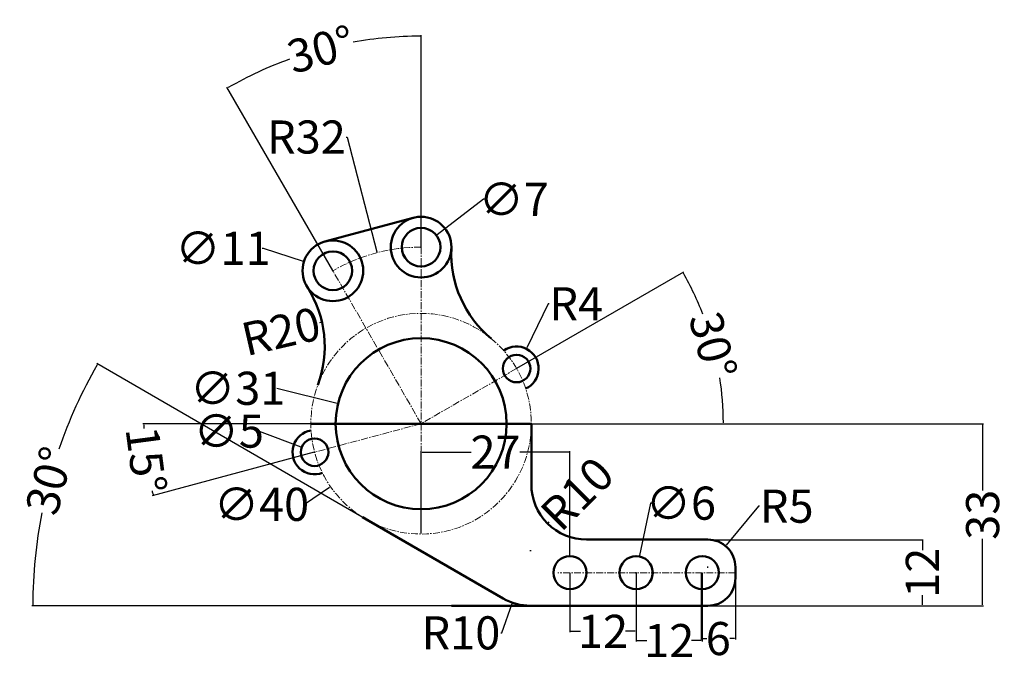
# Model space of a CAD drawing. Units: millimetres. Extents: x 90 to 269, y 31 to 148.
import ezdxf

# ---------------------------------------------------------------- set-up
doc = ezdxf.new("R2010")
doc.units = ezdxf.units.MM
doc.header["$MEASUREMENT"] = 0
doc.linetypes.add('CENTER', pattern=[2, 1.25, -0.25, 0.25, -0.25])
for name, color, linetype, lineweight in [('M-CNTR', 1, 'CENTER', 18), ('M-DIMS', 2, 'Continuous', 25), ('M-OUTL', 7, 'Continuous', 50)]:
    doc.layers.add(name, color=color, linetype=linetype, lineweight=lineweight)
doc.styles.get("Standard").update_dxf_attribs({"font": 'arial.ttf'})
doc.dimstyles.get("Standard").update_dxf_attribs({"dimtxt": 6, "dimasz": 0.18, "dimexe": 0.18, "dimexo": 0.0625, "dimgap": 0.09, "dimtad": 0, "dimtoh": 1, "dimdec": 0, "dimzin": 0, "dimdsep": 46, "dimtxsty": 'Standard', "dimcen": 0.09, "dimadec": 0, "dimazin": 0, "dimtfac": 1, "dimtdec": 0, "dimtofl": 0, "dimtmove": 0, "dimatfit": 3, "dimfxl": 1, "dimtolj": 1, "dimtzin": 0, "dimarcsym": 0})

# ---------------------------------------------------------------- blocks, each defined once
blk = doc.blocks.new('*D1')
at = {"layer": 'Defpoints', "color": 0, "transparency": 16777216}
for p in [(178.24, 74.72), (178.24, 41.72), (264.58, 41.72)]:
    blk.add_point(p, dxfattribs=at)
at = {"layer": 'M-DIMS', "color": 0, "lineweight": -2, "transparency": 16777216}
for p, q in [((178.3, 74.72), (264.76, 74.72)), ((264.58, 74.54), (264.58, 62.61)), ((264.58, 41.9), (264.58, 53.84)), ((178.3, 41.72), (264.76, 41.72))]:
    blk.add_line(p, q, dxfattribs=at)
at = {"layer": 'M-DIMS', "color": 0, "transparency": 16777216}
for points in [[(264.55, 74.54), (264.61, 74.54), (264.58, 74.72)], [(264.55, 41.9), (264.61, 41.9), (264.58, 41.72)]]:
    blk.add_solid(points, dxfattribs=at)
at = {"layer": 'M-DIMS', "color": 0, "transparency": 16777216, "insert": (264.58, 58.22), "char_height": 6, "attachment_point": 5, "rotation": 90}
blk.add_mtext('\\A1;33', dxfattribs=at)
blk = doc.blocks.new('*D2')
at = {"layer": 'Defpoints', "color": 0, "transparency": 16777216}
for p in [(215.42, 53.68), (215.42, 41.72), (253.65, 41.72)]:
    blk.add_point(p, dxfattribs=at)
at = {"layer": 'M-DIMS', "color": 0, "lineweight": -2, "transparency": 16777216}
for p, q in [((215.48, 53.68), (253.83, 53.68)), ((253.65, 53.5), (253.65, 51.77)), ((253.65, 41.9), (253.65, 43.63)), ((215.48, 41.72), (253.83, 41.72))]:
    blk.add_line(p, q, dxfattribs=at)
at = {"layer": 'M-DIMS', "color": 0, "transparency": 16777216}
for points in [[(253.62, 53.5), (253.68, 53.5), (253.65, 53.68)], [(253.62, 41.9), (253.68, 41.9), (253.65, 41.72)]]:
    blk.add_solid(points, dxfattribs=at)
at = {"layer": 'M-DIMS', "color": 0, "transparency": 16777216, "insert": (253.65, 47.7), "char_height": 6, "attachment_point": 5, "rotation": 90}
blk.add_mtext('\\A1;12', dxfattribs=at)
blk = doc.blocks.new('*D3')
at = {"layer": 'Defpoints', "color": 0, "transparency": 16777216}
for p in [(217.93, 52.57), (214.74, 48.72)]:
    blk.add_point(p, dxfattribs=at)
at = {"layer": 'M-DIMS', "color": 0, "lineweight": -2, "transparency": 16777216}
for p, q in [((223.93, 59.77), (218.05, 52.71)), ((224.11, 59.77), (223.93, 59.77)), ((214.65, 48.72), (214.83, 48.72)), ((214.74, 48.63), (214.74, 48.81))]:
    blk.add_line(p, q, dxfattribs=at)
at = {"layer": 'M-DIMS', "color": 0, "transparency": 16777216}
blk.add_solid([(218.03, 52.73), (218.07, 52.69), (217.93, 52.57)], dxfattribs=at)
at = {"layer": 'M-DIMS', "color": 0, "transparency": 16777216, "insert": (229.06, 59.77), "char_height": 6, "attachment_point": 5}
blk.add_mtext('\\A1;R5', dxfattribs=at)
blk = doc.blocks.new('*D4')
at = {"layer": 'Defpoints', "color": 0, "transparency": 16777216}
for p in [(181.82, 88.32), (180.06, 84.72)]:
    blk.add_point(p, dxfattribs=at)
at = {"layer": 'M-DIMS', "color": 0, "lineweight": -2, "transparency": 16777216}
for p, q in [((185.8, 96.45), (181.9, 88.48)), ((185.98, 96.45), (185.8, 96.45)), ((179.97, 84.72), (180.15, 84.72)), ((180.06, 84.63), (180.06, 84.81))]:
    blk.add_line(p, q, dxfattribs=at)
at = {"layer": 'M-DIMS', "color": 0, "transparency": 16777216}
blk.add_solid([(181.87, 88.49), (181.92, 88.46), (181.82, 88.32)], dxfattribs=at)
at = {"layer": 'M-DIMS', "color": 0, "transparency": 16777216, "insert": (190.89, 96.45), "char_height": 6, "attachment_point": 5}
blk.add_mtext('\\A1;R4', dxfattribs=at)
blk = doc.blocks.new('*D5')
at = {"layer": 'Defpoints', "color": 0, "transparency": 16777216}
for p in [(154.75, 105.71), (162.74, 74.72)]:
    blk.add_point(p, dxfattribs=at)
at = {"layer": 'M-DIMS', "color": 0, "lineweight": -2, "transparency": 16777216}
for p, q in [((149.17, 126.68), (149.35, 126.68)), ((149.35, 126.68), (154.71, 105.89)), ((162.65, 74.72), (162.83, 74.72)), ((162.74, 74.63), (162.74, 74.81))]:
    blk.add_line(p, q, dxfattribs=at)
at = {"layer": 'M-DIMS', "color": 0, "transparency": 16777216}
blk.add_solid([(154.74, 105.89), (154.68, 105.88), (154.75, 105.71)], dxfattribs=at)
at = {"layer": 'M-DIMS', "color": 0, "transparency": 16777216, "insert": (141.94, 126.68), "char_height": 6, "attachment_point": 5}
blk.add_mtext('\\A1;R32', dxfattribs=at)
blk = doc.blocks.new('*D6')
at = {"layer": 'Defpoints', "color": 0, "transparency": 16777216}
for p in [(192.74, 63.72), (185.67, 56.65)]:
    blk.add_point(p, dxfattribs=at)
at = {"layer": 'M-DIMS', "color": 0, "lineweight": -2, "transparency": 16777216}
blk.add_line((185.92, 56.91), (185.79, 56.78), dxfattribs=at)
at = {"layer": 'M-DIMS', "color": 0, "transparency": 16777216}
blk.add_solid([(185.77, 56.8), (185.81, 56.76), (185.67, 56.65)], dxfattribs=at)
at = {"layer": 'M-DIMS', "color": 0, "transparency": 16777216, "insert": (191.05, 62.03), "char_height": 6, "attachment_point": 5, "rotation": 45}
blk.add_mtext('\\A1;R10', dxfattribs=at)
blk = doc.blocks.new('*D7')
at = {"layer": 'Defpoints', "color": 0, "transparency": 16777216}
for p in [(182.6, 51.72), (179.3, 42.28)]:
    blk.add_point(p, dxfattribs=at)
at = {"layer": 'M-DIMS', "color": 0, "lineweight": -2, "transparency": 16777216}
for p, q in [((182.6, 51.63), (182.6, 51.81)), ((182.51, 51.72), (182.69, 51.72)), ((177.39, 36.81), (179.24, 42.11)), ((177.21, 36.81), (177.39, 36.81))]:
    blk.add_line(p, q, dxfattribs=at)
at = {"layer": 'M-DIMS', "color": 0, "transparency": 16777216}
blk.add_solid([(179.21, 42.12), (179.27, 42.1), (179.3, 42.28)], dxfattribs=at)
at = {"layer": 'M-DIMS', "color": 0, "transparency": 16777216, "insert": (169.96, 36.81), "char_height": 6, "attachment_point": 5}
blk.add_mtext('\\A1;R10', dxfattribs=at)
blk = doc.blocks.new('*D8')
at = {"layer": 'Defpoints', "color": 0, "transparency": 16777216}
for p in [(189.74, 69.57), (162.74, 54.72), (189.74, 50.72)]:
    blk.add_point(p, dxfattribs=at)
at = {"layer": 'M-DIMS', "color": 0, "lineweight": -2, "transparency": 16777216}
for p, q in [((162.74, 54.79), (162.74, 69.75)), ((189.74, 50.79), (189.74, 69.75)), ((162.92, 69.57), (171.8, 69.57)), ((189.56, 69.57), (180.67, 69.57))]:
    blk.add_line(p, q, dxfattribs=at)
at = {"layer": 'M-DIMS', "color": 0, "transparency": 16777216}
for points in [[(162.92, 69.6), (162.92, 69.54), (162.74, 69.57)], [(189.56, 69.6), (189.56, 69.54), (189.74, 69.57)]]:
    blk.add_solid(points, dxfattribs=at)
at = {"layer": 'M-DIMS', "color": 0, "transparency": 16777216, "insert": (176.24, 69.57), "char_height": 6, "attachment_point": 5}
blk.add_mtext('\\A1;27', dxfattribs=at)
blk = doc.blocks.new('*D9')
at = {"layer": 'Defpoints', "color": 0, "transparency": 16777216}
for p in [(189.74, 47.72), (201.74, 47.72), (201.74, 37.09)]:
    blk.add_point(p, dxfattribs=at)
at = {"layer": 'M-DIMS', "color": 0, "lineweight": -2, "transparency": 16777216}
for p, q in [((189.74, 47.66), (189.74, 36.91)), ((201.74, 47.66), (201.74, 36.91)), ((189.92, 37.09), (191.66, 37.09)), ((201.56, 37.09), (199.81, 37.09))]:
    blk.add_line(p, q, dxfattribs=at)
at = {"layer": 'M-DIMS', "color": 0, "transparency": 16777216}
for points in [[(189.92, 37.12), (189.92, 37.06), (189.74, 37.09)], [(201.56, 37.12), (201.56, 37.06), (201.74, 37.09)]]:
    blk.add_solid(points, dxfattribs=at)
at = {"layer": 'M-DIMS', "color": 0, "transparency": 16777216, "insert": (195.74, 37.09), "char_height": 6, "attachment_point": 5}
blk.add_mtext('\\A1;12', dxfattribs=at)
blk = doc.blocks.new('*D10')
at = {"layer": 'Defpoints', "color": 0, "transparency": 16777216}
for p in [(201.74, 47.72), (213.74, 47.72), (213.74, 35.41)]:
    blk.add_point(p, dxfattribs=at)
at = {"layer": 'M-DIMS', "color": 0, "lineweight": -2, "transparency": 16777216}
for p, q in [((201.74, 47.66), (201.74, 35.23)), ((213.74, 47.66), (213.74, 35.23)), ((201.92, 35.41), (203.66, 35.41)), ((213.56, 35.41), (211.81, 35.41))]:
    blk.add_line(p, q, dxfattribs=at)
at = {"layer": 'M-DIMS', "color": 0, "transparency": 16777216}
for points in [[(201.92, 35.44), (201.92, 35.38), (201.74, 35.41)], [(213.56, 35.44), (213.56, 35.38), (213.74, 35.41)]]:
    blk.add_solid(points, dxfattribs=at)
at = {"layer": 'M-DIMS', "color": 0, "transparency": 16777216, "insert": (207.74, 35.41), "char_height": 6, "attachment_point": 5}
blk.add_mtext('\\A1;12', dxfattribs=at)
blk = doc.blocks.new('*D11')
at = {"layer": 'Defpoints', "color": 0, "transparency": 16777216}
for p in [(213.55, 47.72), (219.74, 47.72), (219.74, 35.78)]:
    blk.add_point(p, dxfattribs=at)
at = {"layer": 'M-DIMS', "color": 0, "lineweight": -2, "transparency": 16777216}
for p, q in [((213.55, 47.66), (213.55, 35.6)), ((219.74, 47.66), (219.74, 35.6)), ((213.73, 35.78), (214.57, 35.78)), ((219.56, 35.78), (218.72, 35.78))]:
    blk.add_line(p, q, dxfattribs=at)
at = {"layer": 'M-DIMS', "color": 0, "transparency": 16777216}
for points in [[(213.73, 35.81), (213.73, 35.75), (213.55, 35.78)], [(219.56, 35.81), (219.56, 35.75), (219.74, 35.78)]]:
    blk.add_solid(points, dxfattribs=at)
at = {"layer": 'M-DIMS', "color": 0, "transparency": 16777216, "insert": (216.64, 35.78), "char_height": 6, "attachment_point": 5}
blk.add_mtext('\\A1;6', dxfattribs=at)
blk = doc.blocks.new('*D12')
at = {"layer": 'Defpoints', "color": 0, "transparency": 16777216}
for p in [(141.5, 104.12), (151.97, 100.75)]:
    blk.add_point(p, dxfattribs=at)
at = {"layer": 'M-DIMS', "color": 0, "lineweight": -2, "transparency": 16777216}
for p, q in [((133.89, 106.51), (134.07, 106.51)), ((134.07, 106.51), (141.33, 104.17)), ((146.65, 102.44), (146.83, 102.44)), ((146.74, 102.35), (146.74, 102.53))]:
    blk.add_line(p, q, dxfattribs=at)
at = {"layer": 'M-DIMS', "color": 0, "transparency": 16777216}
blk.add_solid([(141.34, 104.2), (141.32, 104.14), (141.5, 104.12)], dxfattribs=at)
at = {"layer": 'M-DIMS', "color": 0, "transparency": 16777216, "insert": (126.81, 106.51), "char_height": 6, "attachment_point": 5}
blk.add_mtext('\\A1;∅11', dxfattribs=at)
blk = doc.blocks.new('*D13')
at = {"layer": 'Defpoints', "color": 0, "transparency": 16777216}
for p in [(165.52, 108.85), (159.96, 104.6)]:
    blk.add_point(p, dxfattribs=at)
at = {"layer": 'M-DIMS', "color": 0, "lineweight": -2, "transparency": 16777216}
for p, q in [((174.06, 115.39), (165.66, 108.96)), ((174.24, 115.39), (174.06, 115.39)), ((162.65, 106.72), (162.83, 106.72)), ((162.74, 106.63), (162.74, 106.81))]:
    blk.add_line(p, q, dxfattribs=at)
at = {"layer": 'M-DIMS', "color": 0, "transparency": 16777216}
blk.add_solid([(165.64, 108.98), (165.68, 108.94), (165.52, 108.85)], dxfattribs=at)
at = {"layer": 'M-DIMS', "color": 0, "transparency": 16777216, "insert": (179.56, 115.39), "char_height": 6, "attachment_point": 5}
blk.add_mtext('\\A1;∅7', dxfattribs=at)
blk = doc.blocks.new('*D14')
at = {"layer": 'Defpoints', "color": 0, "transparency": 16777216}
for p in [(141.08, 70.44), (145.75, 68.65)]:
    blk.add_point(p, dxfattribs=at)
at = {"layer": 'M-DIMS', "color": 0, "lineweight": -2, "transparency": 16777216}
for p, q in [((133.21, 73.38), (133.39, 73.38)), ((133.39, 73.38), (140.91, 70.5)), ((143.33, 69.55), (143.51, 69.55)), ((143.42, 69.46), (143.42, 69.64))]:
    blk.add_line(p, q, dxfattribs=at)
at = {"layer": 'M-DIMS', "color": 0, "transparency": 16777216}
blk.add_solid([(140.93, 70.53), (140.9, 70.48), (141.08, 70.44)], dxfattribs=at)
at = {"layer": 'M-DIMS', "color": 0, "transparency": 16777216, "insert": (127.87, 73.38), "char_height": 6, "attachment_point": 5}
blk.add_mtext('\\A1;∅5', dxfattribs=at)
blk = doc.blocks.new('*D15')
at = {"layer": 'Defpoints', "color": 0, "transparency": 16777216}
for p in [(147.68, 78.41), (177.79, 71.03)]:
    blk.add_point(p, dxfattribs=at)
at = {"layer": 'M-DIMS', "color": 0, "lineweight": -2, "transparency": 16777216}
for p, q in [((136.55, 81.14), (147.51, 78.46)), ((162.65, 74.72), (162.83, 74.72)), ((162.74, 74.63), (162.74, 74.81))]:
    blk.add_line(p, q, dxfattribs=at)
at = {"layer": 'M-DIMS', "color": 0, "transparency": 16777216}
blk.add_solid([(147.51, 78.49), (147.5, 78.43), (147.68, 78.41)], dxfattribs=at)
at = {"layer": 'M-DIMS', "color": 0, "transparency": 16777216, "insert": (129.48, 81.14), "char_height": 6, "attachment_point": 5}
blk.add_mtext('\\A1;∅31', dxfattribs=at)
blk = doc.blocks.new('*D16')
at = {"layer": 'Defpoints', "color": 0, "transparency": 16777216}
for p in [(144.75, 93.16), (125.26, 88.7)]:
    blk.add_point(p, dxfattribs=at)
at = {"layer": 'M-DIMS', "color": 0, "lineweight": -2, "transparency": 16777216}
blk.add_line((144.4, 93.08), (144.58, 93.12), dxfattribs=at)
at = {"layer": 'M-DIMS', "color": 0, "transparency": 16777216}
blk.add_solid([(144.57, 93.15), (144.58, 93.09), (144.75, 93.16)], dxfattribs=at)
at = {"layer": 'M-DIMS', "color": 0, "transparency": 16777216, "insert": (137.33, 91.46), "char_height": 6, "attachment_point": 5, "rotation": 12.8998}
blk.add_mtext('\\A1;R20', dxfattribs=at)
blk = doc.blocks.new('*D17')
at = {"layer": 'Defpoints', "color": 0, "transparency": 16777216}
for p in [(179.18, 86.11), (146.29, 63.34)]:
    blk.add_point(p, dxfattribs=at)
at = {"layer": 'M-DIMS', "color": 0, "lineweight": -2, "transparency": 16777216}
for p, q in [((162.65, 74.72), (162.83, 74.72)), ((162.74, 74.63), (162.74, 74.81)), ((141.62, 60.11), (146.14, 63.24)), ((141.44, 60.11), (141.62, 60.11))]:
    blk.add_line(p, q, dxfattribs=at)
at = {"layer": 'M-DIMS', "color": 0, "transparency": 16777216}
blk.add_solid([(146.13, 63.26), (146.16, 63.21), (146.29, 63.34)], dxfattribs=at)
at = {"layer": 'M-DIMS', "color": 0, "transparency": 16777216, "insert": (133.8, 60.11), "char_height": 6, "attachment_point": 5}
blk.add_mtext('\\A1;∅40', dxfattribs=at)
blk = doc.blocks.new('*D18')
at = {"layer": 'Defpoints', "color": 0, "transparency": 16777216}
for p in [(150.54, 143.9), (162.74, 106.72), (146.74, 102.44), (162.74, 74.72), (162.74, 54.72)]:
    blk.add_point(p, dxfattribs=at)
at = {"layer": 'M-DIMS', "color": 0, "lineweight": -2, "transparency": 16777216}
for p, q in [((162.74, 106.79), (162.74, 145.14)), ((146.71, 102.49), (127.53, 135.71))]:
    blk.add_line(p, q, dxfattribs=at)
for start, end in [(90.1468, 100.1216), (109.8784, 119.8532)]:
    blk.add_arc((162.74, 74.72), 70.24, start, end, dxfattribs=at)
at = {"layer": 'M-DIMS', "color": 0, "transparency": 16777216}
for points in [[(162.56, 144.99), (162.56, 144.93), (162.74, 144.96)], [(127.79, 135.62), (127.76, 135.67), (127.62, 135.55)]]:
    blk.add_solid(points, dxfattribs=at)
at = {"layer": 'M-DIMS', "color": 0, "transparency": 16777216, "insert": (144.56, 142.57), "char_height": 6, "attachment_point": 5, "rotation": 15}
blk.add_mtext('\\A1;30°', dxfattribs=at)
blk = doc.blocks.new('*D19')
at = {"layer": 'Defpoints', "color": 0, "transparency": 16777216}
for p in [(97.61, 71.68), (152.13, 57.77), (177.6, 43.06), (168.25, 41.72), (182.6, 41.72)]:
    blk.add_point(p, dxfattribs=at)
at = {"layer": 'M-DIMS', "color": 0, "lineweight": -2, "transparency": 16777216}
for p, q in [((152.07, 57.8), (103.9, 85.61)), ((168.19, 41.72), (92.14, 41.72))]:
    blk.add_line(p, q, dxfattribs=at)
for start, end in [(150.1177, 161.0898), (168.9102, 179.8823)]:
    blk.add_arc((179.92, 41.72), 87.6, start, end, dxfattribs=at)
at = {"layer": 'M-DIMS', "color": 0, "transparency": 16777216}
for points in [[(103.94, 85.38), (104, 85.35), (104.06, 85.52)], [(92.35, 41.9), (92.29, 41.9), (92.32, 41.72)]]:
    blk.add_solid(points, dxfattribs=at)
at = {"layer": 'M-DIMS', "color": 0, "transparency": 16777216, "insert": (95.31, 64.4), "char_height": 6, "attachment_point": 5, "rotation": 75}
blk.add_mtext('\\A1;30°', dxfattribs=at)
blk = doc.blocks.new('*D20')
at = {"layer": 'Defpoints', "color": 0, "transparency": 16777216}
for p in [(142.74, 74.72), (162.74, 74.72), (182.74, 74.72), (112.64, 70.34), (143.42, 69.55)]:
    blk.add_point(p, dxfattribs=at)
at = {"layer": 'M-DIMS', "color": 0, "lineweight": -2, "transparency": 16777216}
for p, q in [((142.67, 74.72), (112.27, 74.72)), ((143.36, 69.53), (113.99, 61.66))]:
    blk.add_line(p, q, dxfattribs=at)
for start, end in [(180.2051, 180.9995), (194.0005, 194.7949)]:
    blk.add_arc((162.74, 74.72), 50.29, start, end, dxfattribs=at)
at = {"layer": 'M-DIMS', "color": 0, "transparency": 16777216}
for points in [[(112.42, 74.54), (112.48, 74.54), (112.45, 74.72)], [(114.15, 61.89), (114.09, 61.88), (114.16, 61.71)]]:
    blk.add_solid(points, dxfattribs=at)
at = {"layer": 'M-DIMS', "color": 0, "transparency": 16777216, "insert": (112.88, 68.16), "char_height": 6, "attachment_point": 5, "rotation": 277.5}
blk.add_mtext('\\A1;15°', dxfattribs=at)
blk = doc.blocks.new('*D21')
at = {"layer": 'Defpoints', "color": 0, "transparency": 16777216}
for p in [(180.06, 84.72), (216.73, 84.24), (142.74, 74.72), (162.74, 74.72), (182.74, 74.72)]:
    blk.add_point(p, dxfattribs=at)
at = {"layer": 'M-DIMS', "color": 0, "lineweight": -2, "transparency": 16777216}
for p, q in [((180.11, 84.76), (210.37, 102.23)), ((182.8, 74.72), (217.74, 74.72))]:
    blk.add_line(p, q, dxfattribs=at)
for start, end in [(21.2551, 29.8119), (0.1881, 8.7449)]:
    blk.add_arc((162.74, 74.72), 54.82, start, end, dxfattribs=at)
at = {"layer": 'M-DIMS', "color": 0, "transparency": 16777216}
for points in [[(210.28, 101.96), (210.33, 101.99), (210.21, 102.14)], [(217.59, 74.9), (217.53, 74.9), (217.56, 74.72)]]:
    blk.add_solid(points, dxfattribs=at)
at = {"layer": 'M-DIMS', "color": 0, "transparency": 16777216, "insert": (215.69, 88.91), "char_height": 6, "attachment_point": 5, "rotation": 285}
blk.add_mtext('\\A1;30°', dxfattribs=at)
blk = doc.blocks.new('*D22')
at = {"layer": 'Defpoints', "color": 0, "transparency": 16777216}
for p in [(202.35, 50.66), (201.13, 44.79)]:
    blk.add_point(p, dxfattribs=at)
at = {"layer": 'M-DIMS', "color": 0, "lineweight": -2, "transparency": 16777216}
for p, q in [((204.36, 60.32), (202.38, 50.84)), ((204.54, 60.32), (204.36, 60.32)), ((201.65, 47.72), (201.83, 47.72)), ((201.74, 47.63), (201.74, 47.81))]:
    blk.add_line(p, q, dxfattribs=at)
at = {"layer": 'M-DIMS', "color": 0, "transparency": 16777216}
blk.add_solid([(202.35, 50.84), (202.41, 50.83), (202.35, 50.66)], dxfattribs=at)
at = {"layer": 'M-DIMS', "color": 0, "transparency": 16777216, "insert": (209.86, 60.32), "char_height": 6, "attachment_point": 5}
blk.add_mtext('\\A1;∅6', dxfattribs=at)

msp = doc.modelspace()

# ---------------------------------------------------------------- linework, layer by layer
at = {"layer": 'M-CNTR'}
for p, q in [((162.74, 74.72), (143.42, 69.55)), ((219.74, 47.72), (187.54, 47.72))]:
    msp.add_line(p, q, dxfattribs=at)
msp.add_lwpolyline([(180.06, 84.72), (162.74, 74.72), (146.74, 102.44, -0.131652), (162.74, 106.72), (162.74, 54.72)], format="xyb", dxfattribs=at)
msp.add_circle((162.74, 74.72), 20, dxfattribs=at)
at = {"layer": 'M-OUTL'}
msp.add_line((145.31, 107.75), (161.31, 112.04), dxfattribs=at)
for points in [[(142.74, 74.72), (182.74, 74.72), (182.74, 63.72, 0.414214), (192.74, 53.72), (214.74, 53.72, -0.414214), (219.74, 48.72), (219.74, 46.72, -0.414214), (214.74, 41.72), (182.6, 41.72)], [(152.13, 57.77), (177.6, 43.06, 0.131652), (182.6, 41.72), (168.25, 41.72)]]:
    msp.add_lwpolyline(points, format="xyb", dxfattribs=at)
msp.add_lwpolyline([(152.35, 57.63), (153.13, 57.18)], dxfattribs=at)
for centre, radius in [((162.74, 106.72), 5.5), ((162.74, 106.72), 3.5), ((146.74, 102.44), 5.5), ((146.74, 102.44), 3.5), ((162.74, 74.72), 15.5), ((180.06, 84.72), 2.5), ((143.42, 69.55), 2.5), ((189.74, 47.72), 3), ((201.74, 47.72), 3), ((213.74, 47.72), 3)]:
    msp.add_circle(centre, radius, dxfattribs=at)
for centre, radius, start, end in [((188.21, 105.56), 20, 177.3924, 230.4434), ((125.26, 88.7), 20, 339.5566, 32.6076), ((180.06, 84.72), 4, 294.2608, 125.7392), ((143.42, 69.55), 4, 99.2608, 290.7392)]:
    msp.add_arc(centre, radius, start, end, dxfattribs=at)

# ---------------------------------------------------------------- dimensions: what is measured, and where the dimension line sits
at = {"layer": 'M-DIMS'}
for base, line1, line2, picture, middle in [((150.54, 143.9), ((162.74, 106.72), (162.74, 54.72)), ((162.74, 74.72), (146.74, 102.44)), '*D18', (144.56, 142.57)), ((216.73, 84.24), ((142.74, 74.72), (182.74, 74.72)), ((180.06, 84.72), (162.74, 74.72)), '*D21', (215.69, 88.91)), ((97.61, 71.68), ((182.6, 41.72), (168.25, 41.72)), ((152.13, 57.77), (177.6, 43.06)), '*D19', (95.31, 64.4)), ((112.64, 70.34), ((162.74, 74.72), (143.42, 69.55)), ((142.74, 74.72), (182.74, 74.72)), '*D20', (112.88, 68.16))]:
    dim = msp.add_angular_dim_2l(base=base, line1=line1, line2=line2, dimstyle='Standard', override={"dimclrd": 0, "dimclre": 0, "dimclrt": 0}, dxfattribs=at)
    dim.commit()
    dim.dimension.update_dxf_attribs({"geometry": picture, "text_midpoint": middle})
for center, mpoint, picture, middle in [((162.74, 74.72), (154.75, 105.71), '*D5', (141.94, 126.68)), ((180.06, 84.72), (181.82, 88.32), '*D4', (190.89, 96.45)), ((125.26, 88.7), (144.75, 93.16), '*D16', (137.33, 91.46)), ((192.74, 63.72), (185.67, 56.65), '*D6', (191.05, 62.03)), ((214.74, 48.72), (217.93, 52.57), '*D3', (229.06, 59.77)), ((182.6, 51.72), (179.3, 42.28), '*D7', (169.96, 36.81))]:
    dim = msp.add_radius_dim(center=center, mpoint=mpoint, dimstyle='Standard', override={"dimclrd": 0, "dimclre": 0, "dimclrt": 0}, dxfattribs=at)
    dim.commit()
    dim.dimension.update_dxf_attribs({"geometry": picture, "text_midpoint": middle, "dimtype": 164})
for p1, p2, picture, middle in [((159.96, 104.6), (165.52, 108.85), '*D13', (179.56, 115.39)), ((151.97, 100.75), (141.5, 104.12), '*D12', (126.81, 106.51)), ((179.18, 86.11), (146.29, 63.34), '*D17', (133.8, 60.11)), ((177.79, 71.03), (147.68, 78.41), '*D15', (136.55, 81.14)), ((145.75, 68.65), (141.08, 70.44), '*D14', (127.87, 73.38)), ((201.13, 44.79), (202.35, 50.66), '*D22', (209.86, 60.32))]:
    dim = msp.add_diameter_dim_2p(p1=p1, p2=p2, dimstyle='Standard', override={"dimclrd": 0, "dimclre": 0, "dimclrt": 0}, dxfattribs=at)
    dim.commit()
    dim.dimension.update_dxf_attribs({"geometry": picture, "text_midpoint": middle, "dimtype": 163})
for base, p1, p2, picture, middle in [((189.74, 69.57), (162.74, 54.72), (189.74, 50.72), '*D8', (176.24, 69.57)), ((201.74, 37.09), (189.74, 47.72), (201.74, 47.72), '*D9', (195.74, 37.09)), ((213.74, 35.41), (201.74, 47.72), (213.74, 47.72), '*D10', (207.74, 35.41)), ((219.74, 35.78), (213.55, 47.72), (219.74, 47.72), '*D11', (216.64, 35.78))]:
    dim = msp.add_linear_dim(base=base, p1=p1, p2=p2, dimstyle='Standard', override={"dimclrd": 0, "dimclre": 0, "dimclrt": 0}, dxfattribs=at)
    dim.commit()
    dim.dimension.update_dxf_attribs({"geometry": picture, "text_midpoint": middle})
for base, p1, p2, picture, middle in [((264.58, 41.72), (178.24, 74.72), (178.24, 41.72), '*D1', (264.58, 58.22)), ((253.65, 41.72), (215.42, 53.68), (215.42, 41.72), '*D2', (253.65, 47.7))]:
    dim = msp.add_linear_dim(base=base, p1=p1, p2=p2, angle=90, dimstyle='Standard', override={"dimclrd": 0, "dimclre": 0, "dimclrt": 0}, dxfattribs=at)
    dim.commit()
    dim.dimension.update_dxf_attribs({"geometry": picture, "text_midpoint": middle})

doc.saveas('drawing.dxf')
